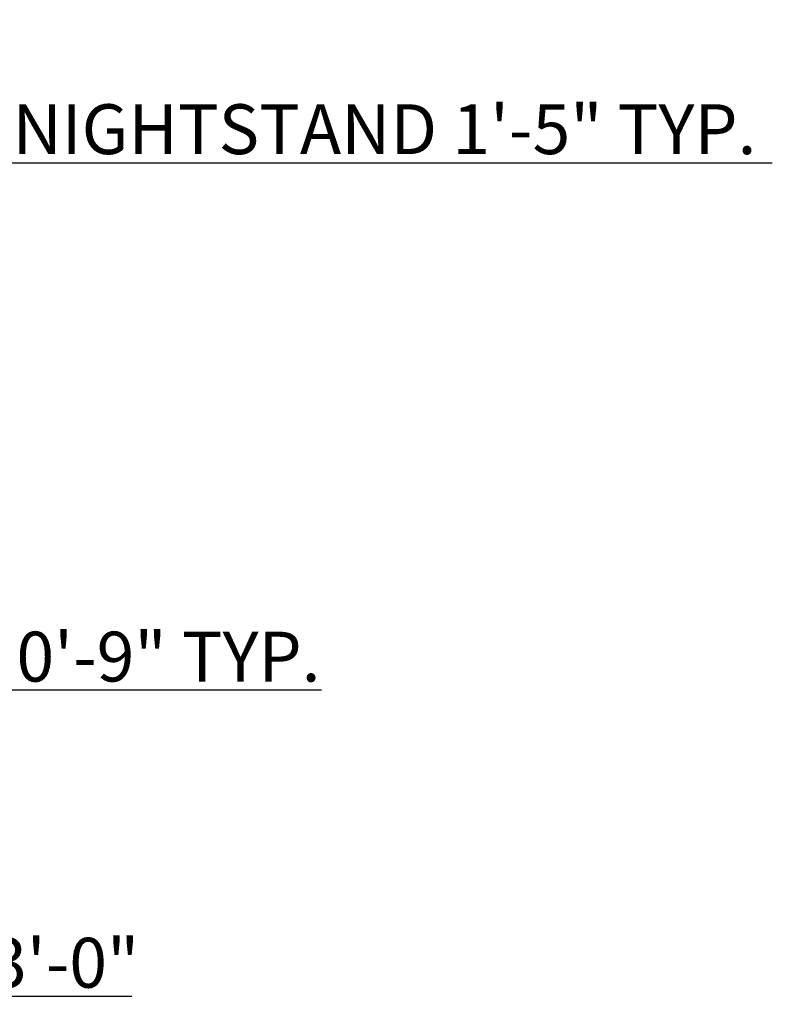
# Model space of a CAD drawing. Units: inches. Extents: x 1383 to 2465, y 1661 to 2415.
# Tile 4 of 4: x 2102 to 2465, y 1680 to 2154. Entities that reach past the tile are written whole.
import ezdxf

# ---------------------------------------------------------------- set-up
doc = ezdxf.new("R2010")
doc.units = ezdxf.units.IN
doc.layers.add('A-ANNO-DIMS', color=2, linetype='Continuous', lineweight=18)
doc.styles.get("Standard").update_dxf_attribs({"font": 'arial.ttf'})
doc.dimstyles.new('ISO-25', dxfattribs={"dimtxt": 24, "dimasz": 24, "dimexe": 1.25, "dimexo": 0.625, "dimtad": 1, "dimdec": 0, "dimlunit": 3, "dimtxsty": 'Standard', "dimcen": 2.5, "dimadec": 0, "dimazin": 0, "dimtfac": 1, "dimtdec": 0, "dimtmove": 0, "dimatfit": 3, "dimfxl": 1, "dimarcsym": 0})

# ---------------------------------------------------------------- blocks, each defined once
blk = doc.blocks.new('*D16')
at = {"layer": 'A-ANNO-DIMS', "color": 0, "lineweight": -2, "transparency": 16777216}
for p, q in [((2025.96, 2087.24), (2025.96, 2084.03)), ((2043.19, 2087.24), (2043.19, 2084.03)), ((2001.96, 2085.28), (1977.96, 2085.28)), ((2025.96, 2085.28), (2043.19, 2085.28)), ((2067.19, 2085.28), (2464.82, 2085.28))]:
    blk.add_line(p, q, dxfattribs=at)
at = {"layer": 'A-ANNO-DIMS', "color": 0, "transparency": 16777216}
for points in [[(2001.96, 2089.28), (2001.96, 2081.28), (2025.96, 2085.28)], [(2067.19, 2089.28), (2067.19, 2081.28), (2043.19, 2085.28)]]:
    blk.add_solid(points, dxfattribs=at)
at = {"layer": 'Defpoints', "color": 0, "transparency": 16777216}
for p in [(2025.96, 2087.86), (2043.19, 2087.86), (2043.19, 2085.28)]:
    blk.add_point(p, dxfattribs=at)
at = {"layer": 'A-ANNO-DIMS', "color": 0, "transparency": 16777216, "insert": (2278.01, 2098.31), "char_height": 24, "attachment_point": 5}
blk.add_mtext('NIGHTSTAND 1\'-5" TYP.', dxfattribs=at)
blk = doc.blocks.new('*D19')
at = {"layer": 'A-ANNO-DIMS', "color": 0, "lineweight": -2, "transparency": 16777216}
for p, q in [((2043.19, 1836.29), (2043.19, 1830.26)), ((2052.19, 1836.29), (2052.19, 1830.26)), ((2019.19, 1831.51), (1995.19, 1831.51)), ((2043.19, 1831.51), (2052.19, 1831.51)), ((2076.19, 1831.51), (2247.74, 1831.51))]:
    blk.add_line(p, q, dxfattribs=at)
at = {"layer": 'A-ANNO-DIMS', "color": 0, "transparency": 16777216}
for points in [[(2019.19, 1835.51), (2019.19, 1827.51), (2043.19, 1831.51)], [(2076.19, 1835.51), (2076.19, 1827.51), (2052.19, 1831.51)]]:
    blk.add_solid(points, dxfattribs=at)
at = {"layer": 'Defpoints', "color": 0, "transparency": 16777216}
for p in [(2043.19, 1836.91), (2052.19, 1836.91), (2052.19, 1831.51)]:
    blk.add_point(p, dxfattribs=at)
at = {"layer": 'A-ANNO-DIMS', "color": 0, "transparency": 16777216, "insert": (2173.96, 1844.39), "char_height": 24, "attachment_point": 5}
blk.add_mtext('0\'-9" TYP.', dxfattribs=at)
blk = doc.blocks.new('*D46')
at = {"layer": 'A-ANNO-DIMS', "color": 0, "lineweight": -2, "transparency": 16777216}
for p, q in [((2007.19, 1786.54), (2007.19, 1682.86)), ((2043.19, 1786.54), (2043.19, 1682.86)), ((1983.19, 1684.11), (1959.19, 1684.11)), ((2007.19, 1684.11), (2043.19, 1684.11)), ((2067.19, 1684.11), (2156.23, 1684.11))]:
    blk.add_line(p, q, dxfattribs=at)
at = {"layer": 'A-ANNO-DIMS', "color": 0, "transparency": 16777216}
for points in [[(1983.19, 1688.11), (1983.19, 1680.11), (2007.19, 1684.11)], [(2067.19, 1688.11), (2067.19, 1680.11), (2043.19, 1684.11)]]:
    blk.add_solid(points, dxfattribs=at)
at = {"layer": 'Defpoints', "color": 0, "transparency": 16777216}
for p in [(2007.19, 1787.16), (2043.19, 1787.16), (2043.19, 1684.11)]:
    blk.add_point(p, dxfattribs=at)
at = {"layer": 'A-ANNO-DIMS', "color": 0, "transparency": 16777216, "insert": (2123.71, 1697), "char_height": 24, "attachment_point": 5}
blk.add_mtext('3\'-0"', dxfattribs=at)

msp = doc.modelspace()

# ---------------------------------------------------------------- dimensions: what is measured, and where the dimension line sits
at = {"layer": 'A-ANNO-DIMS'}
for base, p1, p2, text, picture, middle in [((2043.19, 2085.28), (2025.96, 2087.86), (2043.19, 2087.86), 'NIGHTSTAND <> TYP.', '*D16', (2278.01, 2098.31)), ((2052.19, 1831.51), (2043.19, 1836.91), (2052.19, 1836.91), '<> TYP.', '*D19', (2173.96, 1844.39))]:
    dim = msp.add_linear_dim(base=base, p1=p1, p2=p2, text=text, dimstyle='ISO-25', override={"dimdec": 1, "dimlfac": 1, "dimrnd": 0, "dimzin": 1, "dimdsep": 46, "dimlunit": 4, "dimfrac": 2}, dxfattribs=at)
    dim.commit()
    dim.dimension.update_dxf_attribs({"geometry": picture, "text_midpoint": middle})
dim = msp.add_linear_dim(base=(2043.19, 1684.11), p1=(2007.19, 1787.16), p2=(2043.19, 1787.16), dimstyle='ISO-25', override={"dimdec": 1, "dimlfac": 1, "dimrnd": 0, "dimzin": 1, "dimdsep": 46, "dimlunit": 4, "dimfrac": 2}, dxfattribs=at)
dim.commit()
dim.dimension.update_dxf_attribs({"geometry": '*D46', "text_midpoint": (2123.71, 1697)})

doc.saveas('drawing.dxf')
